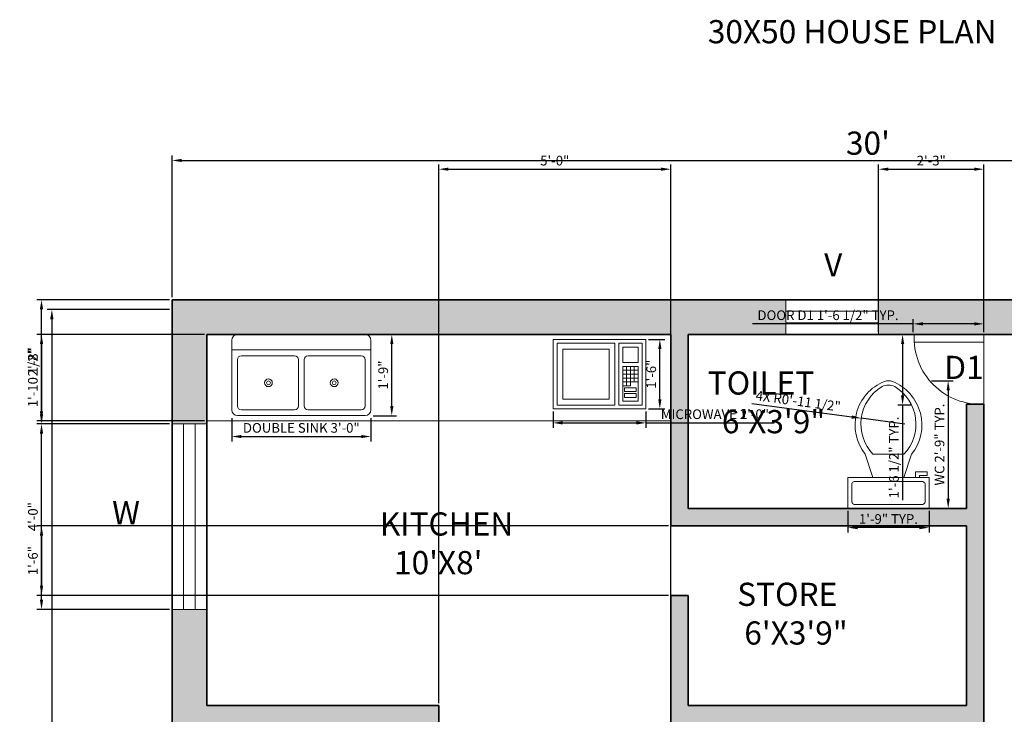
# Model space of a CAD drawing. Units: inches. Extents: x 5030 to 5465, y 5339 to 6047.
# Tile 4 of 5: x 5030 to 5285, y 5867 to 6047. Entities that reach past the tile are written whole.
import ezdxf

# ---------------------------------------------------------------- set-up
doc = ezdxf.new("R2010")
doc.units = ezdxf.units.IN
for name, color, linetype, lineweight in [('A-ANNO-DIMS', 2, 'Continuous', 18), ('A-ANNO-TEXT', 7, 'Continuous', 18), ('A-AREA-IDEN', 7, 'Continuous', 25), ('A-DOOR', 3, 'Continuous', 18), ('A-EQPM', 9, 'Continuous', 18), ('A-FLOR-CASE', 8, 'Continuous', 18), ('A-FLOR-FIXT', 9, 'Continuous', 18), ('A-GLAZ', 4, 'Continuous', 18), ('A-WALL', 7, 'Continuous', 35)]:
    doc.layers.add(name, color=color, linetype=linetype, lineweight=lineweight)
doc.layers.add('A-WALL-PATT', color=149, linetype='Continuous', lineweight=13, true_color=0x444546)
doc.styles.get("Standard").update_dxf_attribs({"font": 'arial.ttf'})
doc.dimstyles.new('ISO-25', dxfattribs={"dimtxt": 2.5, "dimasz": 2.5, "dimexe": 1.25, "dimexo": 0.625, "dimtad": 1, "dimlunit": 3, "dimtxsty": 'Standard', "dimcen": 2.5, "dimadec": 0, "dimazin": 0, "dimtfac": 1, "dimtmove": 0, "dimatfit": 3, "dimfxl": 1, "dimarcsym": 0})

# ---------------------------------------------------------------- blocks, each defined once
blk = doc.blocks.new('Sink-double - 36 in top')
for p, q in [((-18, -4), (18, -4)), ((-0.75, -18.5), (-0.75, -6.5)), ((0.75, -6.5), (0.75, -18.5))]:
    blk.add_line(p, q)
for points in [[(-16.5, 0), (16.5, 0)], [(-18, -19.5), (-18, -1.5)], [(18, -1.5), (18, -19.5)], [(-16.5, -18.5), (-16.5, -6.5)], [(-15.5, -5.5), (-1.75, -5.5)], [(1.75, -5.5), (15.5, -5.5)], [(16.5, -6.5), (16.5, -18.5)], [(-1.75, -19.5), (-15.5, -19.5)], [(15.5, -19.5), (1.75, -19.5)], [(16.5, -21), (-16.5, -21)]]:
    blk.add_lwpolyline(points)
for centre, radius in [((-8.5, -12.5), 1), ((-8.5, -12.5), 0.5), ((8.5, -12.5), 1), ((8.5, -12.5), 0.5)]:
    blk.add_circle(centre, radius)
for centre, radius, start, end in [((-16.5, -1.5), 1.5, 90, 180), ((16.5, -1.5), 1.5, 0, 90), ((-15.5, -6.5), 1, 90, 180), ((-1.75, -6.5), 1, 0, 90), ((1.75, -6.5), 1, 90, 180), ((15.5, -6.5), 1, 0, 90), ((-16.5, -19.5), 1.5, 180, 270), ((-15.5, -18.5), 1, 180, 270), ((-1.75, -18.5), 1, 270, 0), ((1.75, -18.5), 1, 180, 270), ((15.5, -18.5), 1, 270, 0), ((16.5, -19.5), 1.5, 270, 0)]:
    blk.add_arc(centre, radius, start, end)
blk = doc.blocks.new('Microwave')
for p, q in [((19, 7), (19, 11)), ((20, 11), (20, 7)), ((21, 7), (21, 11)), ((18, 10), (22, 10)), ((22, 9), (18, 9)), ((18, 8), (22, 8)), ((22, 7), (18, 7)), ((20, 6), (18, 6)), ((19, 6), (19, 7)), ((20, 7), (20, 6))]:
    blk.add_line(p, q)
for points in [[(0, 0), (0, 18), (24, 18), (24, 0)], [(1, 1), (1, 17), (16, 17), (16, 1)], [(2.5, 2.5), (2.5, 15.5), (14.5, 15.5), (14.5, 2.5)], [(17, 1), (17, 17), (23, 17), (23, 1)], [(18, 12), (18, 16), (22, 16), (22, 12)], [(18, 2), (18, 11), (22, 11), (22, 2)], [(18.5, 4.5), (18.5, 5.5), (21.5, 5.5), (21.5, 4.5)], [(18.5, 3), (18.5, 4), (21.5, 4), (21.5, 3)]]:
    blk.add_lwpolyline(points, close=True)
blk = doc.blocks.new('Toilet - top')
for p, q in [((9.5, -6), (9.5, -2)), ((-10, -8.5), (-8, -8.5)), ((-10, -9.5), (-10, -8.5)), ((-7, -9.5), (-10, -9.5)), ((-8, -8.5), (-8, -8)), ((-7, -8), (-7, -9.5)), ((-4, -8), (-6, -14)), ((4, -8), (6, -14)), ((4, -14), (-4, -14))]:
    blk.add_line(p, q)
blk.add_lwpolyline([(10.5, -8), (10.5, 0), (-10.5, 0), (-10.5, -8)], close=True)
for points in [[(-9.5, -2), (-9.5, -6)], [(8.5, -1), (-8.5, -1)], [(-8.5, -7), (8.5, -7)]]:
    blk.add_lwpolyline(points)
for centre, radius, start, end in [((-8.62, -1.88), 0.884, 81.8699, 188.1301), ((8.62, -1.88), 0.884, 351.8699, 98.1301), ((-8.62, -6.12), 0.884, 171.8699, 278.1301), ((8.62, -6.12), 0.884, 261.8699, 8.1301), ((3.52, -21.58), 12.17, 141.4691, 247.9714), ((4.2, -21.82), 11.33, 136.3677, 238.9468), ((-3.52, -21.58), 12.17, 292.0284, 38.5307), ((-4.2, -21.82), 11.33, 301.053, 43.6321), ((0, -27.88), 4, 245.7318, 294.2682), ((0, -29), 4, 254.8605, 285.1395)]:
    blk.add_arc(centre, radius, start, end)
blk = doc.blocks.new('*D7')
at = {"layer": 'A-ANNO-DIMS', "color": 0, "lineweight": -2, "transparency": 16777216}
for p, q in [((5069.24, 5975.13), (5069.24, 6011.77)), ((5071.74, 6010.52), (5426.74, 6010.52)), ((5429.24, 5975.13), (5429.24, 6011.77))]:
    blk.add_line(p, q, dxfattribs=at)
at = {"layer": 'A-ANNO-DIMS', "color": 0, "transparency": 16777216}
for points in [[(5071.74, 6010.94), (5071.74, 6010.1), (5069.24, 6010.52)], [(5426.74, 6010.94), (5426.74, 6010.1), (5429.24, 6010.52)]]:
    blk.add_solid(points, dxfattribs=at)
at = {"layer": 'Defpoints', "color": 0, "transparency": 16777216}
for p in [(5429.24, 6010.52), (5069.24, 5974.5), (5429.24, 5974.5)]:
    blk.add_point(p, dxfattribs=at)
at = {"layer": 'A-ANNO-DIMS', "color": 0, "transparency": 16777216, "insert": (5249.24, 6014.21), "char_height": 6, "attachment_point": 5}
blk.add_mtext("30'", dxfattribs=at)
blk = doc.blocks.new('*D8')
at = {"layer": 'A-ANNO-DIMS', "color": 0, "lineweight": -2, "transparency": 16777216}
for p, q in [((5068.62, 5971.96), (5036.91, 5971.96)), ((5038.16, 5969.46), (5038.16, 5377)), ((5068.62, 5374.5), (5036.91, 5374.5))]:
    blk.add_line(p, q, dxfattribs=at)
at = {"layer": 'A-ANNO-DIMS', "color": 0, "transparency": 16777216}
for points in [[(5037.74, 5969.46), (5038.58, 5969.46), (5038.16, 5971.96)], [(5037.74, 5377), (5038.58, 5377), (5038.16, 5374.5)]]:
    blk.add_solid(points, dxfattribs=at)
at = {"layer": 'Defpoints', "color": 0, "transparency": 16777216}
for p in [(5069.24, 5971.96), (5038.16, 5374.5), (5069.24, 5374.5)]:
    blk.add_point(p, dxfattribs=at)
at = {"layer": 'A-ANNO-DIMS', "color": 0, "transparency": 16777216, "insert": (5034.47, 5673.23), "char_height": 6, "attachment_point": 5, "rotation": 90}
blk.add_mtext('49\'-9.46"', dxfattribs=at)
blk = doc.blocks.new('VENT-24IN')
for p, q in [((0, 24), (9, 24)), ((3, 24), (3, 0)), ((6, 24), (6, 0)), ((0, 0), (9, 0))]:
    blk.add_line(p, q)
blk = doc.blocks.new('DOOR-SWING-18IN')
for p, q in [((0, 18), (0, 2)), ((18, 2), (0, 2)), ((0, 2), (0, 0)), ((0, 0), (18, 0)), ((18, 0), (18, 2))]:
    blk.add_line(p, q)
blk.add_arc((1, 1), 17.03, 356.6335, 93.3665)
blk = doc.blocks.new('*D21')
at = {"layer": 'A-ANNO-DIMS', "color": 0, "lineweight": -2, "transparency": 16777216}
for p, q in [((5265.67, 5953.55), (5271.25, 5953.55)), ((5270, 5951.05), (5270, 5923)), ((5265.67, 5920.5), (5271.25, 5920.5))]:
    blk.add_line(p, q, dxfattribs=at)
at = {"layer": 'A-ANNO-DIMS', "color": 0, "transparency": 16777216}
for points in [[(5269.59, 5951.05), (5270.42, 5951.05), (5270, 5953.55)], [(5269.59, 5923), (5270.42, 5923), (5270, 5920.5)]]:
    blk.add_solid(points, dxfattribs=at)
at = {"layer": 'Defpoints', "color": 0, "transparency": 16777216}
for p in [(5265.05, 5953.55), (5265.05, 5920.5), (5270, 5920.5)]:
    blk.add_point(p, dxfattribs=at)
at = {"layer": 'A-ANNO-DIMS', "color": 0, "transparency": 16777216, "insert": (5268.09, 5937.03), "char_height": 2.5, "attachment_point": 5, "rotation": 90}
blk.add_mtext('WC 2\'-9" TYP.', dxfattribs=at)
blk = doc.blocks.new('*D22')
at = {"layer": 'A-ANNO-DIMS', "color": 0, "lineweight": -2, "transparency": 16777216}
for p, q in [((5244.05, 5919.88), (5244.05, 5914.3)), ((5265.05, 5919.88), (5265.05, 5914.3)), ((5262.55, 5915.55), (5246.55, 5915.55))]:
    blk.add_line(p, q, dxfattribs=at)
at = {"layer": 'A-ANNO-DIMS', "color": 0, "transparency": 16777216}
for points in [[(5246.55, 5915.96), (5246.55, 5915.13), (5244.05, 5915.55)], [(5262.55, 5915.96), (5262.55, 5915.13), (5265.05, 5915.55)]]:
    blk.add_solid(points, dxfattribs=at)
at = {"layer": 'Defpoints', "color": 0, "transparency": 16777216}
for p in [(5244.05, 5920.5), (5265.05, 5920.5), (5244.05, 5915.55)]:
    blk.add_point(p, dxfattribs=at)
at = {"layer": 'A-ANNO-DIMS', "color": 0, "transparency": 16777216, "insert": (5254.55, 5917.45), "char_height": 2.5, "attachment_point": 5}
blk.add_mtext('1\'-9" TYP.', dxfattribs=at)
blk = doc.blocks.new('*D25')
at = {"layer": 'A-ANNO-DIMS', "color": 0, "lineweight": -2, "transparency": 16777216}
for p, q in [((5260.95, 5968.25), (5219.38, 5968.25)), ((5260.95, 5966.13), (5260.95, 5969.5)), ((5276.74, 5968.25), (5263.45, 5968.25)), ((5279.24, 5966.13), (5279.24, 5969.5))]:
    blk.add_line(p, q, dxfattribs=at)
at = {"layer": 'A-ANNO-DIMS', "color": 0, "transparency": 16777216}
for points in [[(5263.45, 5968.66), (5263.45, 5967.83), (5260.95, 5968.25)], [(5276.74, 5968.66), (5276.74, 5967.83), (5279.24, 5968.25)]]:
    blk.add_solid(points, dxfattribs=at)
at = {"layer": 'Defpoints', "color": 0, "transparency": 16777216}
for p in [(5260.95, 5968.25), (5260.95, 5965.5), (5279.24, 5965.5)]:
    blk.add_point(p, dxfattribs=at)
at = {"layer": 'A-ANNO-DIMS', "color": 0, "transparency": 16777216, "insert": (5238.92, 5970.16), "char_height": 2.5, "attachment_point": 5}
blk.add_mtext('DOOR D1 1\'-6 1/2" TYP.', dxfattribs=at)
blk = doc.blocks.new('*D26')
at = {"layer": 'A-ANNO-DIMS', "color": 0, "lineweight": -2, "transparency": 16777216}
for p, q in [((5260.33, 5965.5), (5256.96, 5965.5)), ((5258.21, 5963), (5258.21, 5949.72)), ((5260.33, 5947.22), (5256.96, 5947.22)), ((5258.21, 5947.22), (5258.21, 5922.64))]:
    blk.add_line(p, q, dxfattribs=at)
at = {"layer": 'A-ANNO-DIMS', "color": 0, "transparency": 16777216}
for points in [[(5257.8, 5963), (5258.63, 5963), (5258.21, 5965.5)], [(5257.8, 5949.72), (5258.63, 5949.72), (5258.21, 5947.22)]]:
    blk.add_solid(points, dxfattribs=at)
at = {"layer": 'Defpoints', "color": 0, "transparency": 16777216}
for p in [(5260.95, 5965.5), (5258.21, 5947.22), (5260.95, 5947.22)]:
    blk.add_point(p, dxfattribs=at)
at = {"layer": 'A-ANNO-DIMS', "color": 0, "transparency": 16777216, "insert": (5256.29, 5933.68), "char_height": 2.5, "attachment_point": 5, "rotation": 90}
blk.add_mtext('1\'-6 1/2" TYP.', dxfattribs=at)
blk = doc.blocks.new('*D29')
at = {"layer": 'A-ANNO-DIMS', "color": 0, "lineweight": -2, "transparency": 16777216}
for p, q in [((5084.69, 5943.88), (5084.69, 5937.85)), ((5120.69, 5943.88), (5120.69, 5937.85)), ((5087.19, 5939.1), (5118.19, 5939.1))]:
    blk.add_line(p, q, dxfattribs=at)
at = {"layer": 'A-ANNO-DIMS', "color": 0, "transparency": 16777216}
for points in [[(5087.19, 5939.52), (5087.19, 5938.69), (5084.69, 5939.1)], [(5118.19, 5939.52), (5118.19, 5938.69), (5120.69, 5939.1)]]:
    blk.add_solid(points, dxfattribs=at)
at = {"layer": 'Defpoints', "color": 0, "transparency": 16777216}
for p in [(5084.69, 5944.5), (5120.69, 5944.5), (5120.69, 5939.1)]:
    blk.add_point(p, dxfattribs=at)
at = {"layer": 'A-ANNO-DIMS', "color": 0, "transparency": 16777216, "insert": (5102.69, 5941.02), "char_height": 2.5, "attachment_point": 5}
blk.add_mtext('DOUBLE SINK 3\'-0"', dxfattribs=at)
blk = doc.blocks.new('*D30')
at = {"layer": 'A-ANNO-DIMS', "color": 0, "lineweight": -2, "transparency": 16777216}
for p, q in [((5121.31, 5965.5), (5127.34, 5965.5)), ((5126.09, 5947), (5126.09, 5963)), ((5121.31, 5944.5), (5127.34, 5944.5))]:
    blk.add_line(p, q, dxfattribs=at)
at = {"layer": 'A-ANNO-DIMS', "color": 0, "transparency": 16777216}
for points in [[(5125.67, 5963), (5126.51, 5963), (5126.09, 5965.5)], [(5125.67, 5947), (5126.51, 5947), (5126.09, 5944.5)]]:
    blk.add_solid(points, dxfattribs=at)
at = {"layer": 'Defpoints', "color": 0, "transparency": 16777216}
for p in [(5120.69, 5965.5), (5126.09, 5965.5), (5120.69, 5944.5)]:
    blk.add_point(p, dxfattribs=at)
at = {"layer": 'A-ANNO-DIMS', "color": 0, "transparency": 16777216, "insert": (5124.19, 5955), "char_height": 2.5, "attachment_point": 5, "rotation": 90}
blk.add_mtext('1\'-9"', dxfattribs=at)
blk = doc.blocks.new('*D31')
at = {"layer": 'A-ANNO-DIMS', "color": 0, "lineweight": -2, "transparency": 16777216}
for p, q in [((5167.82, 5945.6), (5167.82, 5941.38)), ((5191.82, 5945.6), (5191.82, 5941.38)), ((5170.32, 5942.63), (5189.32, 5942.63)), ((5191.82, 5942.63), (5225, 5942.63))]:
    blk.add_line(p, q, dxfattribs=at)
at = {"layer": 'A-ANNO-DIMS', "color": 0, "transparency": 16777216}
for points in [[(5170.32, 5943.05), (5170.32, 5942.21), (5167.82, 5942.63)], [(5189.32, 5943.05), (5189.32, 5942.21), (5191.82, 5942.63)]]:
    blk.add_solid(points, dxfattribs=at)
at = {"layer": 'Defpoints', "color": 0, "transparency": 16777216}
for p in [(5167.82, 5946.23), (5191.82, 5946.23), (5191.82, 5942.63)]:
    blk.add_point(p, dxfattribs=at)
at = {"layer": 'A-ANNO-DIMS', "color": 0, "transparency": 16777216, "insert": (5209.66, 5944.55), "char_height": 2.5, "attachment_point": 5}
blk.add_mtext('MICROWAVE 2\'-0"', dxfattribs=at)
blk = doc.blocks.new('*D32')
at = {"layer": 'A-ANNO-DIMS', "color": 0, "lineweight": -2, "transparency": 16777216}
for p, q in [((5192.45, 5964.23), (5196.67, 5964.23)), ((5195.42, 5948.73), (5195.42, 5961.73)), ((5192.45, 5946.23), (5196.67, 5946.23))]:
    blk.add_line(p, q, dxfattribs=at)
at = {"layer": 'A-ANNO-DIMS', "color": 0, "transparency": 16777216}
for points in [[(5195.01, 5961.73), (5195.84, 5961.73), (5195.42, 5964.23)], [(5195.01, 5948.73), (5195.84, 5948.73), (5195.42, 5946.23)]]:
    blk.add_solid(points, dxfattribs=at)
at = {"layer": 'Defpoints', "color": 0, "transparency": 16777216}
for p in [(5191.82, 5964.23), (5195.42, 5964.23), (5191.82, 5946.23)]:
    blk.add_point(p, dxfattribs=at)
at = {"layer": 'A-ANNO-DIMS', "color": 0, "transparency": 16777216, "insert": (5193.52, 5955.23), "char_height": 2.5, "attachment_point": 5, "rotation": 90}
blk.add_mtext('1\'-6"', dxfattribs=at)
blk = doc.blocks.new('*D38')
at = {"layer": 'A-ANNO-DIMS', "color": 0, "lineweight": -2, "transparency": 16777216}
for p, q in [((5068.62, 5942.38), (5034.24, 5942.38)), ((5035.49, 5896.88), (5035.49, 5939.88)), ((5068.62, 5894.38), (5034.24, 5894.38))]:
    blk.add_line(p, q, dxfattribs=at)
at = {"layer": 'A-ANNO-DIMS', "color": 0, "transparency": 16777216}
for points in [[(5035.07, 5939.88), (5035.91, 5939.88), (5035.49, 5942.38)], [(5035.07, 5896.88), (5035.91, 5896.88), (5035.49, 5894.38)]]:
    blk.add_solid(points, dxfattribs=at)
at = {"layer": 'Defpoints', "color": 0, "transparency": 16777216}
for p in [(5035.49, 5942.38), (5069.24, 5942.38), (5069.24, 5894.38)]:
    blk.add_point(p, dxfattribs=at)
at = {"layer": 'A-ANNO-DIMS', "color": 0, "transparency": 16777216, "insert": (5033.59, 5918.38), "char_height": 2.5, "attachment_point": 5, "rotation": 90}
blk.add_mtext('4\'-0"', dxfattribs=at)
blk = doc.blocks.new('*D49')
at = {"layer": 'A-ANNO-DIMS', "color": 0, "lineweight": -2, "transparency": 16777216}
for p, q in [((5068.62, 5974.5), (5034.24, 5974.5)), ((5035.49, 5944.88), (5035.49, 5972)), ((5068.62, 5942.38), (5034.24, 5942.38))]:
    blk.add_line(p, q, dxfattribs=at)
at = {"layer": 'A-ANNO-DIMS', "color": 0, "transparency": 16777216}
for points in [[(5035.07, 5972), (5035.91, 5972), (5035.49, 5974.5)], [(5035.07, 5944.88), (5035.91, 5944.88), (5035.49, 5942.38)]]:
    blk.add_solid(points, dxfattribs=at)
at = {"layer": 'Defpoints', "color": 0, "transparency": 16777216}
for p in [(5035.49, 5974.5), (5069.24, 5974.5), (5069.24, 5942.38)]:
    blk.add_point(p, dxfattribs=at)
at = {"layer": 'A-ANNO-DIMS', "color": 0, "transparency": 16777216, "insert": (5033.59, 5958.44), "char_height": 2.5, "attachment_point": 5, "rotation": 90}
blk.add_mtext('2\'-8"', dxfattribs=at)
blk = doc.blocks.new('*D50')
at = {"layer": 'A-ANNO-DIMS', "color": 0, "lineweight": -2, "transparency": 16777216}
for p, q in [((5252, 5966.13), (5252, 6009.5)), ((5254.5, 6008.25), (5276.74, 6008.25)), ((5279.24, 5966.13), (5279.24, 6009.5))]:
    blk.add_line(p, q, dxfattribs=at)
at = {"layer": 'A-ANNO-DIMS', "color": 0, "transparency": 16777216}
for points in [[(5254.5, 6008.67), (5254.5, 6007.84), (5252, 6008.25)], [(5276.74, 6008.67), (5276.74, 6007.84), (5279.24, 6008.25)]]:
    blk.add_solid(points, dxfattribs=at)
at = {"layer": 'Defpoints', "color": 0, "transparency": 16777216}
for p in [(5279.24, 6008.25), (5252, 5965.5), (5279.24, 5965.5)]:
    blk.add_point(p, dxfattribs=at)
at = {"layer": 'A-ANNO-DIMS', "color": 0, "transparency": 16777216, "insert": (5265.62, 6010.16), "char_height": 2.5, "attachment_point": 5}
blk.add_mtext('2\'-3"', dxfattribs=at)
blk = doc.blocks.new('*D52')
at = {"layer": 'A-ANNO-DIMS', "color": 0, "lineweight": -2, "transparency": 16777216}
for p, q in [((5077.62, 5965.5), (5034.24, 5965.5)), ((5035.49, 5963), (5035.49, 5945.65)), ((5077.62, 5943.15), (5034.24, 5943.15))]:
    blk.add_line(p, q, dxfattribs=at)
at = {"layer": 'A-ANNO-DIMS', "color": 0, "transparency": 16777216}
for points in [[(5035.07, 5963), (5035.91, 5963), (5035.49, 5965.5)], [(5035.07, 5945.65), (5035.91, 5945.65), (5035.49, 5943.15)]]:
    blk.add_solid(points, dxfattribs=at)
at = {"layer": 'Defpoints', "color": 0, "transparency": 16777216}
for p in [(5078.24, 5965.5), (5035.49, 5943.15), (5078.24, 5943.15)]:
    blk.add_point(p, dxfattribs=at)
at = {"layer": 'A-ANNO-DIMS', "color": 0, "transparency": 16777216, "insert": (5033.57, 5954.33), "char_height": 2.5, "attachment_point": 5, "rotation": 90}
blk.add_mtext('1\'-10 1/2"', dxfattribs=at)
blk = doc.blocks.new('*D53')
at = {"layer": 'A-ANNO-DIMS', "color": 0, "lineweight": -2, "transparency": 16777216}
for p, q in [((5197.62, 5916), (5034.24, 5916)), ((5035.49, 5913.5), (5035.49, 5900.5)), ((5197.62, 5898), (5034.24, 5898))]:
    blk.add_line(p, q, dxfattribs=at)
at = {"layer": 'A-ANNO-DIMS', "color": 0, "transparency": 16777216}
for points in [[(5035.07, 5913.5), (5035.91, 5913.5), (5035.49, 5916)], [(5035.07, 5900.5), (5035.91, 5900.5), (5035.49, 5898)]]:
    blk.add_solid(points, dxfattribs=at)
at = {"layer": 'Defpoints', "color": 0, "transparency": 16777216}
for p in [(5198.24, 5916), (5035.49, 5898), (5198.24, 5898)]:
    blk.add_point(p, dxfattribs=at)
at = {"layer": 'A-ANNO-DIMS', "color": 0, "transparency": 16777216, "insert": (5033.59, 5907), "char_height": 2.5, "attachment_point": 5, "rotation": 90}
blk.add_mtext('1\'-6"', dxfattribs=at)
blk = doc.blocks.new('*D54')
at = {"layer": 'A-ANNO-DIMS', "color": 0, "lineweight": -2, "transparency": 16777216}
for p, q in [((5138.24, 5870.13), (5138.24, 6009.5)), ((5140.74, 6008.25), (5195.74, 6008.25)), ((5198.24, 5865.63), (5198.24, 6009.5))]:
    blk.add_line(p, q, dxfattribs=at)
at = {"layer": 'A-ANNO-DIMS', "color": 0, "transparency": 16777216}
for points in [[(5140.74, 6008.67), (5140.74, 6007.84), (5138.24, 6008.25)], [(5195.74, 6008.67), (5195.74, 6007.84), (5198.24, 6008.25)]]:
    blk.add_solid(points, dxfattribs=at)
at = {"layer": 'Defpoints', "color": 0, "transparency": 16777216}
for p in [(5198.24, 6008.25), (5138.24, 5869.5), (5198.24, 5865)]:
    blk.add_point(p, dxfattribs=at)
at = {"layer": 'A-ANNO-DIMS', "color": 0, "transparency": 16777216, "insert": (5168.24, 6010.15), "char_height": 2.5, "attachment_point": 5}
blk.add_mtext('5\'-0"', dxfattribs=at)
blk = doc.blocks.new('*D69')
at = {"layer": 'A-ANNO-DIMS', "color": 0, "lineweight": -2, "transparency": 16777216}
for p, q in [((5219.25, 5947.63), (5245.04, 5944.16)), ((5258.75, 5942.32), (5247.52, 5943.83))]:
    blk.add_line(p, q, dxfattribs=at)
at = {"layer": 'A-ANNO-DIMS', "color": 0, "transparency": 16777216}
blk.add_solid([(5245.1, 5944.58), (5244.99, 5943.75), (5247.52, 5943.83)], dxfattribs=at)
at = {"layer": 'Defpoints', "color": 0, "transparency": 16777216}
for p in [(5247.52, 5943.83), (5258.75, 5942.32)]:
    blk.add_point(p, dxfattribs=at)
at = {"layer": 'A-ANNO-DIMS', "color": 0, "transparency": 16777216, "insert": (5231.16, 5947.96), "char_height": 2.5, "attachment_point": 5, "rotation": 352.3435}
blk.add_mtext('4X R0\'-11 1/2"', dxfattribs=at)

msp = doc.modelspace()

# ---------------------------------------------------------------- hatches: boundary and pattern name
at = {"layer": 'A-WALL-PATT'}
h = msp.add_hatch(color=256, dxfattribs=at)
h.dxf.hatch_style = 1
h.paths.add_polyline_path([(5227.999, 5974.503), (5069.24, 5974.503), (5069.24, 5942.38), (5078.24, 5942.38), (5078.24, 5965.503), (5198.24, 5965.503), (5198.24, 5916.003), (5274.74, 5916.003), (5274.74, 5869.503), (5202.74, 5869.503), (5202.74, 5898.003), (5198.24, 5898.003), (5198.24, 5865.003), (5274.74, 5865.003), (5274.74, 5817.003, -0.0121933), (5276.74, 5817.003), (5279.24, 5817.003), (5279.24, 5947.503, -0.0293864), (5277.24, 5947.503), (5274.74, 5947.503), (5274.74, 5920.503), (5202.74, 5920.503), (5202.74, 5965.503), (5227.999, 5965.503)])
h.paths.add_polyline_path([(5078.24, 5894.38), (5069.24, 5894.38), (5069.24, 5845.837), (5078.24, 5845.837), (5078.24, 5865.003), (5138.24, 5865.003), (5138.24, 5869.503), (5078.24, 5869.503)], flags=17)
h.paths.add_polyline_path([(5316.341, 5974.503), (5251.999, 5974.503), (5251.999, 5965.503), (5279.24, 5965.503), (5316.341, 5965.503)])
h.paths.add_polyline_path([(5429.24, 5974.503), (5376.341, 5974.503), (5376.341, 5965.503), (5420.24, 5965.503), (5420.24, 5904.986), (5429.24, 5904.986)])
h.paths.add_polyline_path([(5429.24, 5844.986), (5420.24, 5844.986), (5420.24, 5773.503), (5279.24, 5773.503), (5279.24, 5775.003), (5274.74, 5775.003), (5274.74, 5644.503), (5279.24, 5644.503), (5279.24, 5686.503), (5279.24, 5769.003), (5420.24, 5769.003), (5420.24, 5738.095), (5429.24, 5738.095)])
h.paths.add_polyline_path([(5429.24, 5678.095), (5420.24, 5678.095), (5420.24, 5649.003), (5321.24, 5649.003), (5321.24, 5646.503, -0.0121933), (5321.24, 5644.503), (5343.74, 5644.503), (5343.74, 5614.503, -0.0293864), (5345.74, 5614.503), (5348.24, 5614.503), (5348.24, 5644.503), (5420.24, 5644.503), (5420.24, 5636.807), (5429.24, 5636.807)])
h.paths.add_polyline_path([(5429.24, 5612.807), (5420.24, 5612.807), (5420.24, 5596.503), (5321.24, 5596.503, -0.0121933), (5321.24, 5594.503), (5321.24, 5592.003), (5420.24, 5592.003), (5420.24, 5566.431), (5429.24, 5566.431)])
h.paths.add_polyline_path([(5429.24, 5506.431), (5420.24, 5506.431), (5420.24, 5472.003), (5279.24, 5472.003), (5279.24, 5596.503), (5126.24, 5596.503), (5126.24, 5589.503, -0.0106371), (5126.24, 5587.503), (5274.74, 5587.503), (5274.74, 5468.003), (5420.24, 5468.003), (5420.24, 5452.536), (5429.24, 5452.536)])
h.paths.add_polyline_path([(5429.24, 5392.536), (5420.24, 5392.536), (5420.24, 5383.503), (5274.74, 5383.503), (5274.74, 5374.503), (5429.24, 5374.503)])
h.paths.add_polyline_path([(5101.667, 5383.503), (5078.24, 5383.503), (5078.24, 5683.152), (5069.24, 5683.152), (5069.24, 5374.503), (5101.667, 5374.503)])
h.paths.add_polyline_path([(5078.24, 5770.503), (5221.745, 5770.503), (5221.745, 5775.003), (5078.24, 5775.003), (5078.24, 5785.837), (5069.24, 5785.837), (5069.24, 5743.152), (5078.24, 5743.152)])
h.paths.add_polyline_path([(5274.74, 5379.003), (5101.667, 5379.003), (5101.667, 5374.503), (5274.74, 5374.503)])

# ---------------------------------------------------------------- linework, layer by layer
at = {"layer": 'A-FLOR-CASE'}
msp.add_line((5078.24, 5943.147), (5198.24, 5943.147), dxfattribs=at)
at = {"layer": 'A-GLAZ'}
for p, q in [((5069.24, 5942.38), (5078.24, 5942.38)), ((5072.24, 5894.38), (5072.24, 5942.38)), ((5075.24, 5894.38), (5075.24, 5942.38)), ((5069.24, 5894.38), (5078.24, 5894.38))]:
    msp.add_line(p, q, dxfattribs=at)
at = {"layer": 'A-WALL'}
for p, q in [((5069.24, 5974.503), (5429.24, 5974.503)), ((5069.24, 5374.503), (5069.24, 5974.503)), ((5078.24, 5965.503), (5198.24, 5965.503)), ((5078.24, 5869.503), (5078.24, 5965.503)), ((5198.24, 5916.003), (5198.24, 5965.503)), ((5202.74, 5965.503), (5279.24, 5965.503)), ((5202.74, 5920.503), (5202.74, 5965.503)), ((5279.24, 5965.503), (5420.24, 5965.503)), ((5274.74, 5947.503), (5279.24, 5947.503)), ((5274.74, 5920.503), (5274.74, 5947.503)), ((5279.24, 5817.003), (5279.24, 5947.503)), ((5202.74, 5920.503), (5274.74, 5920.503)), ((5198.24, 5916.003), (5274.74, 5916.003)), ((5274.74, 5869.503), (5274.74, 5916.003)), ((5198.24, 5865.003), (5198.24, 5898.003)), ((5198.24, 5898.003), (5202.74, 5898.003)), ((5202.74, 5869.503), (5202.74, 5898.003)), ((5078.24, 5869.503), (5138.24, 5869.503)), ((5138.24, 5869.503), (5138.24, 5865.003)), ((5202.74, 5869.503), (5274.74, 5869.503))]:
    msp.add_line(p, q, dxfattribs=at)

# ---------------------------------------------------------------- block references
at = {"layer": 'A-DOOR', "rotation": 180}
msp.add_blockref('DOOR-SWING-18IN', (5279.24, 5965.503), dxfattribs=at)
at = {"layer": 'A-EQPM'}
msp.add_blockref('Microwave', (5167.822, 5946.23), dxfattribs=at)
at = {"layer": 'A-FLOR-FIXT'}
msp.add_blockref('Sink-double - 36 in top', (5102.689, 5965.503), dxfattribs=at)
at = {"layer": 'A-FLOR-FIXT', "rotation": 180}
msp.add_blockref('Toilet - top', (5254.548, 5920.503), dxfattribs=at)
at = {"layer": 'A-GLAZ', "rotation": 89.9999999999986}
msp.add_blockref('VENT-24IN', (5252, 5965.503), dxfattribs=at)

# ---------------------------------------------------------------- texts
at = {"layer": 'A-ANNO-TEXT', "char_height": 6, "attachment_point": 1}
for s, width, heights, insert in [('30X50 HOUSE PLAN', 116.1833, [25.553], (5207.839, 6046.818)), ('V ', 54.21026, [0], (5237.906, 5986.529)), ('D1 ', 54.21026, [0], (5268.996, 5959.979)), ('W ', 54.21026, [0], (5053.75, 5922.413))]:
    msp.add_mtext_dynamic_manual_height_columns(s, width=width, gutter_width=12.5, heights=heights, dxfattribs=dict(at, insert=insert))
at = {"layer": 'A-AREA-IDEN', "char_height": 6, "attachment_point": 1}
for s, insert in [(' {\\fTimes New Roman|b0|i0|c0|p18; TOILET\\P    6\'X3\'9"}', (5204.136, 5955.95)), (" {\\fTimes New Roman|b0|i0|c0|p18;KITCHEN\\P   10'X8'}", (5121.167, 5919.481)), (' {\\fTimes New Roman|b0|i0|c0|p18; STORE\\P   6\'X3\'9"}', (5211.769, 5901.288))]:
    msp.add_mtext_dynamic_manual_height_columns(s, width=54.21026, gutter_width=12.5, heights=[0], dxfattribs=dict(at, insert=insert))

# ---------------------------------------------------------------- dimensions: what is measured, and where the dimension line sits
at = {"layer": 'A-ANNO-DIMS'}
for base, p1, p2, override, picture, middle in [((5429.24, 6010.52), (5069.24, 5974.503), (5429.24, 5974.503), {"dimtxt": 6, "dimclrd": 0, "dimclre": 0, "dimclrt": 0}, '*D7', (5249.24, 6014.211)), ((5198.24, 6008.253), (5138.24, 5869.503), (5198.24, 5865.003), {"dimdec": 1, "dimlfac": 1, "dimrnd": 0, "dimzin": 1, "dimdsep": 46, "dimlunit": 4, "dimfrac": 2}, '*D54', (5168.24, 6010.155)), ((5279.24, 6008.253), (5251.999, 5965.503), (5279.24, 5965.503), {"dimdec": 1, "dimlfac": 1, "dimrnd": 0, "dimzin": 1, "dimdsep": 46, "dimlunit": 4, "dimfrac": 2}, '*D50', (5265.62, 6010.155))]:
    dim = msp.add_linear_dim(base=base, p1=p1, p2=p2, dimstyle='ISO-25', override=override, dxfattribs=at)
    dim.commit()
    dim.dimension.update_dxf_attribs({"geometry": picture, "text_midpoint": middle})
for base, p1, p2, angle, text, picture, middle in [((5260.955, 5968.246), (5279.24, 5965.503), (5260.955, 5965.503), 180, 'DOOR D1 <> TYP.', '*D25', (5238.918, 5970.164)), ((5258.212, 5947.217), (5260.955, 5965.503), (5260.955, 5947.217), 270, '<> TYP.', '*D26', (5256.294, 5933.678)), ((5270.005, 5920.503), (5265.048, 5953.549), (5265.048, 5920.503), 270, 'WC <> TYP.', '*D21', (5268.087, 5937.026)), ((5244.048, 5915.546), (5265.048, 5920.503), (5244.048, 5920.503), 180, '<> TYP.', '*D22', (5254.548, 5917.448))]:
    dim = msp.add_linear_dim(base=base, p1=p1, p2=p2, angle=angle, text=text, dimstyle='ISO-25', override={"dimdec": 1, "dimlfac": 1, "dimrnd": 0, "dimzin": 1, "dimdsep": 46, "dimlunit": 4, "dimfrac": 2}, dxfattribs=at)
    dim.commit()
    dim.dimension.update_dxf_attribs({"geometry": picture, "text_midpoint": middle})
for base, p1, p2, override, picture, middle in [((5035.49, 5974.503), (5069.24, 5942.38), (5069.24, 5974.503), {"dimdec": 1, "dimlfac": 1, "dimrnd": 0, "dimzin": 1, "dimdsep": 46, "dimlunit": 4, "dimfrac": 2}, '*D49', (5033.589, 5958.441)), ((5038.161, 5374.503), (5069.24, 5971.965), (5069.24, 5374.503), {"dimtxt": 6, "dimclrd": 0, "dimclre": 0, "dimclrt": 0}, '*D8', (5034.472, 5673.234)), ((5035.49, 5943.147), (5078.24, 5965.503), (5078.24, 5943.147), {"dimdec": 1, "dimlfac": 1, "dimrnd": 0, "dimzin": 1, "dimdsep": 46, "dimlunit": 4, "dimfrac": 2}, '*D52', (5033.573, 5954.325)), ((5126.089, 5965.503), (5120.689, 5944.503), (5120.689, 5965.503), {"dimdec": 1, "dimlfac": 1, "dimrnd": 0, "dimzin": 1, "dimdsep": 46, "dimlunit": 4, "dimfrac": 2}, '*D30', (5124.188, 5955.003)), ((5195.422, 5964.23), (5191.822, 5946.23), (5191.822, 5964.23), {"dimdec": 1, "dimlfac": 1, "dimrnd": 0, "dimzin": 1, "dimdsep": 46, "dimlunit": 4, "dimfrac": 2}, '*D32', (5193.521, 5955.23)), ((5035.49, 5942.38), (5069.24, 5894.38), (5069.24, 5942.38), {"dimdec": 1, "dimlfac": 1, "dimrnd": 0, "dimzin": 1, "dimdsep": 46, "dimlunit": 4, "dimfrac": 2}, '*D38', (5033.589, 5918.38)), ((5035.49, 5898.003), (5198.24, 5916.003), (5198.24, 5898.003), {"dimdec": 1, "dimlfac": 1, "dimrnd": 0, "dimzin": 1, "dimdsep": 46, "dimlunit": 4, "dimfrac": 2}, '*D53', (5033.589, 5907.003))]:
    dim = msp.add_linear_dim(base=base, p1=p1, p2=p2, angle=90, dimstyle='ISO-25', override=override, dxfattribs=at)
    dim.commit()
    dim.dimension.update_dxf_attribs({"geometry": picture, "text_midpoint": middle})
dim = msp.add_radius_dim(center=(5258.748, 5942.321), mpoint=(5247.519, 5943.83), text='4X <>', dimstyle='ISO-25', override={"dimdec": 1, "dimlfac": 1, "dimrnd": 0, "dimzin": 1, "dimdsep": 46, "dimlunit": 4, "dimfrac": 2}, dxfattribs=at)
dim.commit()
dim.dimension.update_dxf_attribs({"geometry": '*D69', "text_midpoint": (5231.16, 5947.964)})
for base, p1, p2, text, picture, middle in [((5120.689, 5939.103), (5084.689, 5944.503), (5120.689, 5944.503), 'DOUBLE SINK <>', '*D29', (5102.689, 5941.022)), ((5191.822, 5942.63), (5167.822, 5946.23), (5191.822, 5946.23), 'MICROWAVE <>', '*D31', (5209.661, 5944.548))]:
    dim = msp.add_linear_dim(base=base, p1=p1, p2=p2, text=text, dimstyle='ISO-25', override={"dimdec": 1, "dimlfac": 1, "dimrnd": 0, "dimzin": 1, "dimdsep": 46, "dimlunit": 4, "dimfrac": 2}, dxfattribs=at)
    dim.commit()
    dim.dimension.update_dxf_attribs({"geometry": picture, "text_midpoint": middle})

doc.saveas('drawing.dxf')
